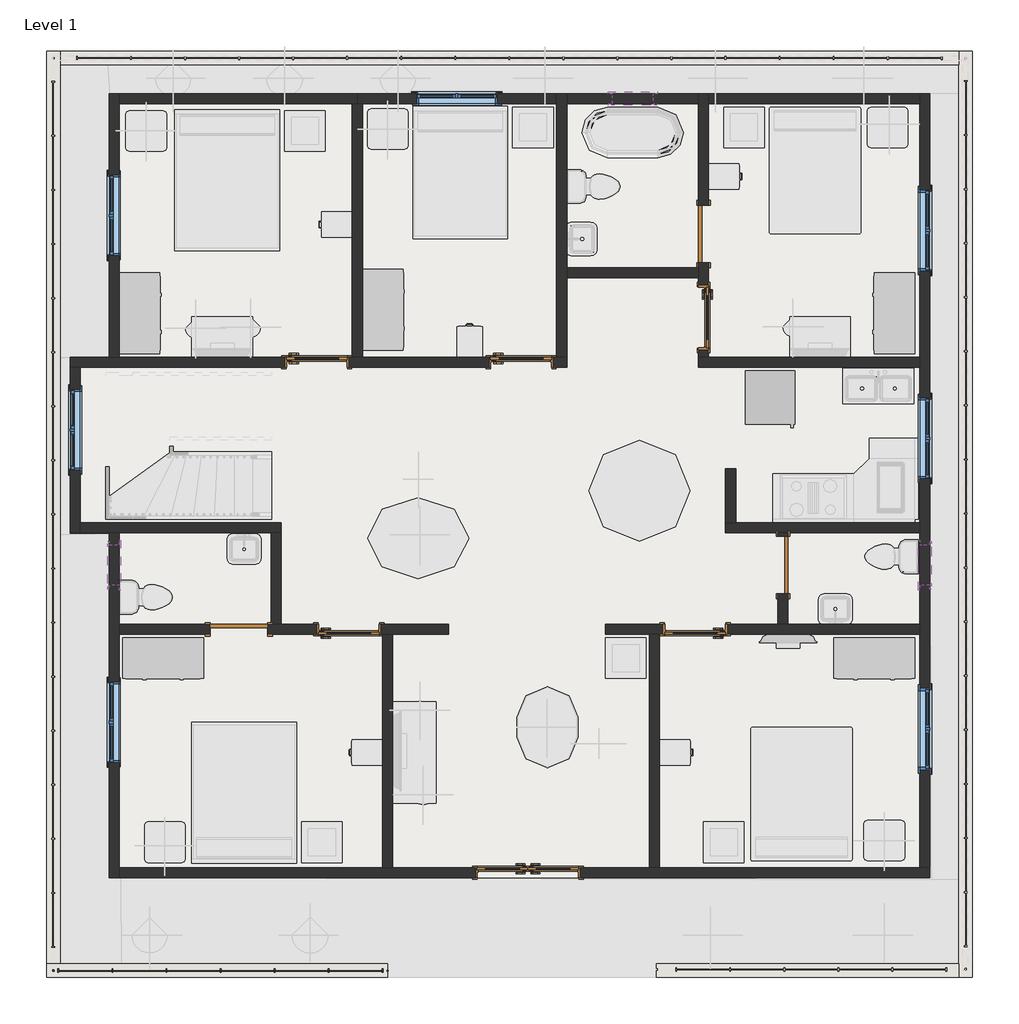
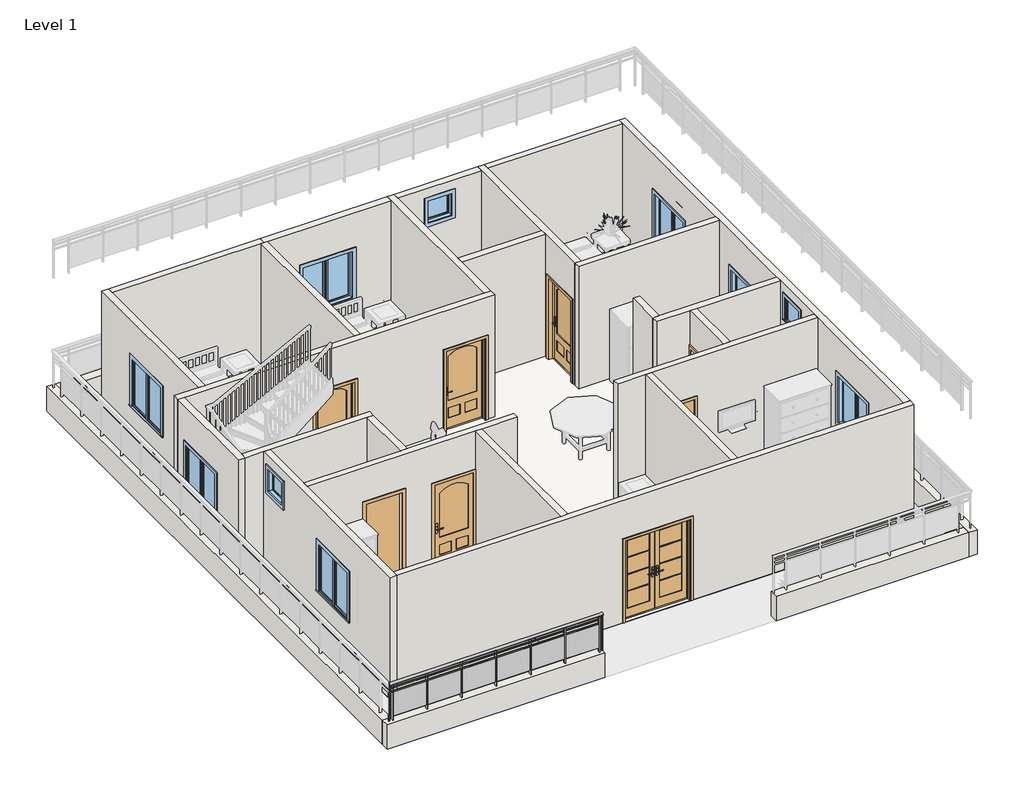
# One storey, part 1 of 5: 29 walls, 10 windows, 9 doors, 1 railing, 1 slab.
"""IFC4 building model written with IfcOpenShell, lengths in millimetres."""

from ifc_helpers import new_model, si_unit, point, frame, origin, origin_with_axes, place, context, project, spatial, polyline, ellipse_curve, trimmed, outline, extrude, faceted_brep, transform, mapped, element, save
from ifc_brep_helpers import plane_surface, extruded_surface, advanced_brep
from components import door_5d363d20, door_808aeb8e, door_94998e6c, door_99d96fc5, door_b6e9fca3, window_be30da88, window_3d781103

model = new_model("IFC4")

# Units and contexts
model_context = context("Model", 3, world=origin())
ifc_project = project(units=[si_unit("LENGTHUNIT", "METRE", prefix="MILLI")], contexts=[model_context])

# Site, building, storey
site = spatial("IfcSite", under=ifc_project)
building = spatial("IfcBuilding", under=site)
storey = spatial("IfcBuildingStorey", under=building, Name="Level 1", Elevation=0.0)

# Doors
placement = place(None, origin())
door_shape = door_5d363d20(model_context)
element("IfcDoor", 1, ObjectType="36\" x 80\"", at=placement, inside=storey, context=model_context, shape_type="MappedRepresentation", body=[
    mapped(door_shape, transform((-7516.6434666, 9773.3466937, 0.0), x_axis=(-1.0, 0.0, 0.0), y_axis=(0.0, -1.0, 0.0), z_axis=(0.0, 0.0, 1.0))),
])
element("IfcDoor", 2, ObjectType="36\" x 80\"", at=placement, inside=storey, context=model_context, shape_type="MappedRepresentation", body=[
    mapped(door_shape, transform((-4443.2434666, 9773.3466937, 0.0), x_axis=(-1.0, 0.0, 0.0), y_axis=(0.0, -1.0, 0.0), z_axis=(0.0, 0.0, 1.0))),
])
element("IfcDoor", 3, ObjectType="36\" x 80\"", at=placement, inside=storey, context=model_context, shape_type="MappedRepresentation", body=[
    mapped(door_shape, transform((-1696.8684666, 10443.2716937, 0.0), x_axis=(0.0, 1.0, 0.0), y_axis=(-1.0, 0.0, 0.0), z_axis=(0.0, 0.0, 1.0))),
])
element("IfcDoor", 4, ObjectType="36\" x 80\"", at=placement, inside=storey, context=model_context, shape_type="MappedRepresentation", body=[
    mapped(door_shape, transform((-1827.0434666, 5753.7966937, 0.0), x_axis=(1.0, 0.0, 0.0), y_axis=(0.0, 1.0, 0.0), z_axis=(0.0, 0.0, 1.0))),
])
door_2_shape = door_808aeb8e(model_context)
element("IfcDoor", 5, ObjectType="36\" x 80\"", at=placement, inside=storey, context=model_context, shape_type="MappedRepresentation", body=[
    mapped(door_2_shape, transform((-7034.0434666, 5753.7966937, 0.0), x_axis=(-1.0, 0.0, 0.0), y_axis=(0.0, -1.0, 0.0), z_axis=(0.0, 0.0, 1.0))),
])
door_3_shape = door_94998e6c(model_context)
element("IfcDoor", 6, ObjectType="Door-Exterior-Double-Full Glass-Wood_Clad : 60\" x 80\"", at=placement, inside=storey, context=model_context, shape_type="MappedRepresentation", body=[
    mapped(door_3_shape, transform((-4341.6434666, 2102.5466937, 0.0), x_axis=(1.0, 0.0, 0.0), y_axis=(0.0, 1.0, 0.0), z_axis=(0.0, 0.0, 1.0))),
])
door_4_shape = door_99d96fc5(model_context)
element("IfcDoor", 7, ObjectType="Single-Flush : 34\" x 84\"", at=placement, inside=storey, context=model_context, shape_type="MappedRepresentation", body=[
    mapped(door_4_shape, transform((-1700.0434666, 11700.5716937, 0.0), x_axis=(0.0, -1.0, 0.0), y_axis=(1.0, 0.0, 0.0), z_axis=(0.0, 0.0, 1.0))),
])
element("IfcDoor", 8, ObjectType="Single-Flush : 34\" x 84\"", at=placement, inside=storey, context=model_context, shape_type="MappedRepresentation", body=[
    mapped(door_4_shape, transform((-506.2434666, 6722.1716937, 0.0), x_axis=(0.0, 1.0, 0.0), y_axis=(-1.0, 0.0, 0.0), z_axis=(0.0, 0.0, 1.0))),
])
door_5_shape = door_b6e9fca3(model_context)
element("IfcDoor", 9, ObjectType="Single-Flush : 34\" x 84\"", at=placement, inside=storey, context=model_context, shape_type="MappedRepresentation", body=[
    mapped(door_5_shape, transform((-8685.0434666, 5756.9716937, 0.0), x_axis=(1.0, 0.0, 0.0), y_axis=(0.0, 1.0, 0.0), z_axis=(0.0, 0.0, 1.0))),
])

# Railing
element("IfcRailing", 10, ObjectType="Glass Panel - Bottom Fill", at=placement, inside=storey, context=model_context, shape_type="SolidModel", body=[
    advanced_brep(
    [(-6449.8434666, 588.0716937, 1524.0), (-6449.8434666, 664.2716937, 1524.0), (-11479.0434666, 588.0716937, 1524.0), (-11479.0434666, 664.2716937, 1524.0)],
    [
        (0, 1, ellipse_curve(frame((-6449.8434666, 626.1716937, 1524.0), z_axis=(1.0, 0.0, 0.0), x_axis=(0.0, 1.0, 0.0)), 38.1, 28.575)),
        (1, 0, ellipse_curve(frame((-6449.8434666, 626.1716937, 1524.0), z_axis=(1.0, 0.0, 0.0), x_axis=(0.0, 1.0, 0.0)), 38.1, 28.575)),
        (2, 3, ellipse_curve(frame((-11479.0434666, 626.1716937, 1524.0), z_axis=(-1.0, 0.0, 0.0), x_axis=(0.0, 1.0, 0.0)), 38.1, 28.575)),
        (3, 2, ellipse_curve(frame((-11479.0434666, 626.1716937, 1524.0), z_axis=(-1.0, 0.0, 0.0), x_axis=(0.0, 1.0, 0.0)), 38.1, 28.575)),
        (0, 2),
        (3, 1),
    ],
    [
        plane_surface(frame((-6449.8434666, 626.1716937, 1524.0), z_axis=(1.0, 0.0, 0.0), x_axis=(0.0, -1.0, 0.0))),
        plane_surface(frame((-11479.0434666, 626.1716937, 1524.0), z_axis=(-1.0, 0.0, 0.0), x_axis=(0.0, -1.0, 0.0))),
        extruded_surface(trimmed(ellipse_curve(frame((-11479.0434666, 626.1716937, 1524.0), z_axis=(1.0, 0.0, 0.0), x_axis=(0.0, 1.0, 0.0)), 38.1, 28.575), [point((-11479.0434666, 588.0716937, 1524.0))], [point((-11479.0434666, 664.2716937, 1524.0))], True, "CARTESIAN"), (5029.2, 0.0, 0.0), 5029.2),
        extruded_surface(trimmed(ellipse_curve(frame((-11479.0434666, 626.1716937, 1524.0), z_axis=(1.0, 0.0, 0.0), x_axis=(0.0, 1.0, 0.0)), 38.1, 28.575), [point((-11479.0434666, 664.2716937, 1524.0))], [point((-11479.0434666, 588.0716937, 1524.0))], True, "CARTESIAN"), (5029.2, 0.0, 0.0), 5029.2),
    ],
    [
        (0, [[1, 2]]),
        (1, [[3, 4]]),
        (2, [[-1, 5, -4, 6]]),
        (3, [[-2, -6, -3, -5]]),
    ],
),
    extrude(outline(polyline([(-6449.8434666, 638.8716937), (-6449.8434666, 613.4716937), (-11479.0434666, 613.4716937), (-11479.0434666, 638.8716937), (-6449.8434666, 638.8716937)])), frame((0.0, 0.0, 1409.7), z_axis=(0.0, 0.0, 1.0), x_axis=(1.0, 0.0, 0.0)), (0.0, 0.0, 1.0), 25.4),
    extrude(outline(polyline([(-6449.8434666, 638.8716937), (-6449.8434666, 613.4716937), (-11479.0434666, 613.4716937), (-11479.0434666, 638.8716937), (-6449.8434666, 638.8716937)])), frame((0.0, 0.0, 1308.1), z_axis=(0.0, 0.0, 1.0), x_axis=(1.0, 0.0, 0.0)), (0.0, 0.0, 1.0), 25.4),
    extrude(outline(polyline([(-11396.4934666, 651.5716937), (-11396.4934666, 600.7716937), (-11409.1934666, 600.7716937), (-11409.1934666, 651.5716937), (-11396.4934666, 651.5716937)])), frame((0.0, 0.0, 609.6), z_axis=(0.0, 0.0, 1.0), x_axis=(1.0, 0.0, 0.0)), (0.0, 0.0, 1.0), 885.6788223),
    extrude(outline(polyline([(-10590.0434666, 619.6365367), (-11402.8434666, 619.6365367), (-11402.8434666, 625.9865367), (-10590.0434666, 625.9865367), (-10590.0434666, 619.6365367)])), frame((0.0, 0.0, 711.2), z_axis=(0.0, 0.0, 1.0), x_axis=(1.0, 0.0, 0.0)), (0.0, 0.0, 1.0), 596.9),
    extrude(outline(polyline([(-10583.6934666, 651.5716937), (-10583.6934666, 600.7716937), (-10596.3934666, 600.7716937), (-10596.3934666, 651.5716937), (-10583.6934666, 651.5716937)])), frame((0.0, 0.0, 609.6), z_axis=(0.0, 0.0, 1.0), x_axis=(1.0, 0.0, 0.0)), (0.0, 0.0, 1.0), 885.6788223),
    extrude(outline(polyline([(-9777.2434666, 619.6365367), (-10590.0434666, 619.6365367), (-10590.0434666, 625.9865367), (-9777.2434666, 625.9865367), (-9777.2434666, 619.6365367)])), frame((0.0, 0.0, 711.2), z_axis=(0.0, 0.0, 1.0), x_axis=(1.0, 0.0, 0.0)), (0.0, 0.0, 1.0), 596.9),
    extrude(outline(polyline([(-9770.8934666, 651.5716937), (-9770.8934666, 600.7716937), (-9783.5934666, 600.7716937), (-9783.5934666, 651.5716937), (-9770.8934666, 651.5716937)])), frame((0.0, 0.0, 609.6), z_axis=(0.0, 0.0, 1.0), x_axis=(1.0, 0.0, 0.0)), (0.0, 0.0, 1.0), 885.6788223),
    extrude(outline(polyline([(-8964.4434666, 619.6365367), (-9777.2434666, 619.6365367), (-9777.2434666, 625.9865367), (-8964.4434666, 625.9865367), (-8964.4434666, 619.6365367)])), frame((0.0, 0.0, 711.2), z_axis=(0.0, 0.0, 1.0), x_axis=(1.0, 0.0, 0.0)), (0.0, 0.0, 1.0), 596.9),
    extrude(outline(polyline([(-8958.0934666, 651.5716937), (-8958.0934666, 600.7716937), (-8970.7934666, 600.7716937), (-8970.7934666, 651.5716937), (-8958.0934666, 651.5716937)])), frame((0.0, 0.0, 609.6), z_axis=(0.0, 0.0, 1.0), x_axis=(1.0, 0.0, 0.0)), (0.0, 0.0, 1.0), 885.6788223),
    extrude(outline(polyline([(-8151.6434666, 619.6365367), (-8964.4434666, 619.6365367), (-8964.4434666, 625.9865367), (-8151.6434666, 625.9865367), (-8151.6434666, 619.6365367)])), frame((0.0, 0.0, 711.2), z_axis=(0.0, 0.0, 1.0), x_axis=(1.0, 0.0, 0.0)), (0.0, 0.0, 1.0), 596.9),
    extrude(outline(polyline([(-8145.2934666, 651.5716937), (-8145.2934666, 600.7716937), (-8157.9934666, 600.7716937), (-8157.9934666, 651.5716937), (-8145.2934666, 651.5716937)])), frame((0.0, 0.0, 609.6), z_axis=(0.0, 0.0, 1.0), x_axis=(1.0, 0.0, 0.0)), (0.0, 0.0, 1.0), 885.6788223),
    extrude(outline(polyline([(-7338.8434666, 619.6365367), (-8151.6434666, 619.6365367), (-8151.6434666, 625.9865367), (-7338.8434666, 625.9865367), (-7338.8434666, 619.6365367)])), frame((0.0, 0.0, 711.2), z_axis=(0.0, 0.0, 1.0), x_axis=(1.0, 0.0, 0.0)), (0.0, 0.0, 1.0), 596.9),
    extrude(outline(polyline([(-7332.4934666, 651.5716937), (-7332.4934666, 600.7716937), (-7345.1934666, 600.7716937), (-7345.1934666, 651.5716937), (-7332.4934666, 651.5716937)])), frame((0.0, 0.0, 609.6), z_axis=(0.0, 0.0, 1.0), x_axis=(1.0, 0.0, 0.0)), (0.0, 0.0, 1.0), 885.6788223),
    extrude(outline(polyline([(-6526.0434666, 619.6365367), (-7338.8434666, 619.6365367), (-7338.8434666, 625.9865367), (-6526.0434666, 625.9865367), (-6526.0434666, 619.6365367)])), frame((0.0, 0.0, 711.2), z_axis=(0.0, 0.0, 1.0), x_axis=(1.0, 0.0, 0.0)), (0.0, 0.0, 1.0), 596.9),
    extrude(outline(polyline([(-6519.6934666, 651.5716937), (-6519.6934666, 600.7716937), (-6532.3934666, 600.7716937), (-6532.3934666, 651.5716937), (-6519.6934666, 651.5716937)])), frame((0.0, 0.0, 609.6), z_axis=(0.0, 0.0, 1.0), x_axis=(1.0, 0.0, 0.0)), (0.0, 0.0, 1.0), 885.6788223),
    extrude(outline(polyline([(-11466.3434666, 635.6966937), (-11466.3434666, 616.6466937), (-11485.3934666, 616.6466937), (-11485.3934666, 635.6966937), (-11466.3434666, 635.6966937)])), frame((0.0, 0.0, 609.6), z_axis=(0.0, 0.0, 1.0), x_axis=(1.0, 0.0, 0.0)), (0.0, 0.0, 1.0), 885.6788223),
    extrude(outline(polyline([(-6443.4934666, 635.6966937), (-6443.4934666, 616.6466937), (-6462.5434666, 616.6466937), (-6462.5434666, 635.6966937), (-6443.4934666, 635.6966937)])), frame((0.0, 0.0, 609.6), z_axis=(0.0, 0.0, 1.0), x_axis=(1.0, 0.0, 0.0)), (0.0, 0.0, 1.0), 885.6788223),
])

# Slab
element("IfcSlab", 11, ObjectType="Generic - 12\"", at=placement, inside=storey, context=model_context, shape_type="SweptSolid", body=[
    extrude(outline(polyline([(1703.5565334, 13808.7716937), (1703.5565334, 2023.1716937), (-10640.8434666, 2023.1716937), (-10640.8434666, 7204.7716937), (-11225.0434666, 7204.7716937), (-11225.0434666, 9846.3716937), (-10640.8434666, 9846.3716937), (-10640.8434666, 13808.7716937), (1703.5565334, 13808.7716937)])), frame((0.0, 0.0, -304.8), z_axis=(0.0, 0.0, 1.0), x_axis=(1.0, 0.0, 0.0)), (0.0, 0.0, 1.0), 304.8),
])

# Walls
element("IfcWall", 12, ObjectType="Generic - 5'", at=placement, inside=storey, context=model_context, shape_type="Brep", body=[
    faceted_brep([(2135.3565334, 14443.7716937, 0.0), (2135.3565334, 14240.5716937, 0.0), (2135.3565334, 727.7716937, 0.0), (2135.3565334, 524.5716937, 0.0), (2135.3565334, 524.5716937, 609.6), (2135.3565334, 727.7716937, 609.6), (2135.3565334, 14240.5716937, 609.6), (2135.3565334, 14443.7716937, 609.6), (2338.5565334, 14443.7716937, 0.0), (2338.5565334, 14443.7716937, 609.6), (2338.5565334, 524.5716937, 609.6), (2338.5565334, 524.5716937, 0.0)], [[[0, 1, 2, 3, 4, 5, 6, 7]], [[8, 9, 10, 11]], [[3, 2, 1, 0, 8, 11]], [[7, 6, 5, 4, 10, 9]], [[4, 3, 11, 10]], [[0, 7, 9, 8]]]),
])
element("IfcWall", 13, ObjectType="Generic - 5'", at=placement, inside=storey, context=model_context, shape_type="SweptSolid", body=[
    extrude(outline(polyline([(-2411.2434666, 727.7716937), (2135.3565334, 727.7716937), (2135.3565334, 524.5716937), (-2411.2434666, 524.5716937), (-2411.2434666, 727.7716937)])), origin_with_axes(), (0.0, 0.0, 1.0), 609.6),
])
element("IfcWall", 14, ObjectType="Generic - 5'", at=placement, inside=storey, context=model_context, shape_type="Brep", body=[
    faceted_brep([(-11377.4434666, 727.7716937, 0.0), (-11377.4434666, 14240.5716937, 0.0), (-11377.4434666, 14443.7716937, 0.0), (-11377.4434666, 14443.7716937, 609.6), (-11377.4434666, 14240.5716937, 609.6), (-11377.4434666, 727.7716937, 609.6), (-11580.6434666, 727.7716937, 0.0), (-11580.6434666, 727.7716937, 609.6), (-11580.6434666, 14443.7716937, 609.6), (-11580.6434666, 14443.7716937, 0.0)], [[[0, 1, 2, 3, 4, 5]], [[6, 7, 8, 9]], [[2, 1, 0, 6, 9]], [[5, 4, 3, 8, 7]], [[0, 5, 7, 6]], [[3, 2, 9, 8]]]),
])
element("IfcWall", 15, ObjectType="Generic - 5'", at=placement, inside=storey, context=model_context, shape_type="SweptSolid", body=[
    extrude(outline(polyline([(2135.3565334, 14240.5716937), (-11377.4434666, 14240.5716937), (-11377.4434666, 14443.7716937), (2135.3565334, 14443.7716937), (2135.3565334, 14240.5716937)])), origin_with_axes(), (0.0, 0.0, 1.0), 609.6),
])
element("IfcWall", 16, ObjectType="Generic - 5'", at=placement, inside=storey, context=model_context, shape_type="Brep", body=[
    faceted_brep([(-6449.8434666, 727.7716937, 0.0), (-11377.4434666, 727.7716937, 0.0), (-11580.6434666, 727.7716937, 0.0), (-11580.6434666, 727.7716937, 609.6), (-11377.4434666, 727.7716937, 609.6), (-6449.8434666, 727.7716937, 609.6), (-6449.8434666, 524.5716937, 0.0), (-6449.8434666, 524.5716937, 609.6), (-11580.6434666, 524.5716937, 609.6), (-11580.6434666, 524.5716937, 0.0)], [[[0, 1, 2, 3, 4, 5]], [[6, 7, 8, 9]], [[2, 1, 0, 6, 9]], [[5, 4, 3, 8, 7]], [[0, 5, 7, 6]], [[3, 2, 9, 8]]]),
])
element("IfcWall", 17, ObjectType="INNER WALL 6\"", at=placement, inside=storey, context=model_context, shape_type="Brep", body=[
    faceted_brep([(-11225.0434666, 9693.9716937, 3048.0), (-11225.0434666, 9693.9716937, 0.0), (-11072.6434666, 9693.9716937, 0.0), (-7999.2434666, 9693.9716937, 0.0), (-7999.2434666, 9693.9716937, 2057.4), (-7034.0434666, 9693.9716937, 2057.4), (-7034.0434666, 9693.9716937, 0.0), (-4925.8434666, 9693.9716937, 0.0), (-4925.8434666, 9693.9716937, 2057.4), (-3960.6434666, 9693.9716937, 2057.4), (-3960.6434666, 9693.9716937, 0.0), (-3757.4434666, 9693.9716937, 0.0), (-3757.4434666, 9693.9716937, 3048.0), (-11072.6434666, 9693.9716937, 3048.0), (-11225.0434666, 9846.3716937, 0.0), (-11225.0434666, 9846.3716937, 3048.0), (-10640.8434666, 9846.3716937, 3048.0), (-10488.4434666, 9846.3716937, 3048.0), (-6983.2434666, 9846.3716937, 3048.0), (-6830.8434666, 9846.3716937, 3048.0), (-3909.8434666, 9846.3716937, 3048.0), (-3757.4434666, 9846.3716937, 3048.0), (-3757.4434666, 9846.3716937, 0.0), (-3909.8434666, 9846.3716937, 0.0), (-3960.6434666, 9846.3716937, 0.0), (-3960.6434666, 9846.3716937, 2057.4), (-4925.8434666, 9846.3716937, 2057.4), (-4925.8434666, 9846.3716937, 0.0), (-6830.8434666, 9846.3716937, 0.0), (-6983.2434666, 9846.3716937, 0.0), (-7034.0434666, 9846.3716937, 0.0), (-7034.0434666, 9846.3716937, 2057.4), (-7999.2434666, 9846.3716937, 2057.4), (-7999.2434666, 9846.3716937, 0.0), (-10488.4434666, 9846.3716937, 0.0), (-10640.8434666, 9846.3716937, 0.0)], [[[0, 1, 2, 3, 4, 5, 6, 7, 8, 9, 10, 11, 12, 13]], [[14, 15, 16, 17, 18, 19, 20, 21, 22, 23, 24, 25, 26, 27, 28, 29, 30, 31, 32, 33, 34, 35]], [[1, 14, 35, 34, 33, 3, 2]], [[22, 11, 10, 24, 23]], [[6, 30, 29, 28, 27, 7]], [[1, 0, 15, 14]], [[12, 11, 22, 21]], [[32, 4, 3, 33]], [[4, 32, 31, 5]], [[5, 31, 30, 6]], [[26, 8, 7, 27]], [[8, 26, 25, 9]], [[9, 25, 24, 10]], [[0, 13, 12, 21, 20, 19, 18, 17, 16, 15]]]),
])
element("IfcWall", 18, ObjectType="INNER WALL 6\"", at=placement, inside=storey, context=model_context, shape_type="Brep", body=[
    faceted_brep([(-10488.4434666, 13656.3716937, 0.0), (-6983.2434666, 13656.3716937, 0.0), (-6907.0434666, 13656.3716937, 0.0), (-6907.0434666, 13656.3716937, 3048.0), (-6983.2434666, 13656.3716937, 3048.0), (-10488.4434666, 13656.3716937, 3048.0), (-10488.4434666, 13808.7716937, 0.0), (-10488.4434666, 13808.7716937, 3048.0), (-6907.0434666, 13808.7716937, 3048.0), (-6907.0434666, 13808.7716937, 0.0)], [[[0, 1, 2, 3, 4, 5]], [[6, 7, 8, 9]], [[2, 1, 0, 6, 9]], [[3, 2, 9, 8]], [[0, 5, 7, 6]], [[5, 4, 3, 8, 7]]]),
])
element("IfcWall", 19, ObjectType="INNER WALL 6\"", at=placement, inside=storey, context=model_context, shape_type="Brep", body=[
    faceted_brep([(-10640.8434666, 13808.7716937, 0.0), (-10640.8434666, 9846.3716937, 0.0), (-10640.8434666, 9846.3716937, 3048.0), (-10640.8434666, 13808.7716937, 3048.0), (-10640.8434666, 12589.5716937, 2133.6), (-10640.8434666, 11370.3716937, 2133.6), (-10640.8434666, 11370.3716937, 914.4), (-10640.8434666, 12589.5716937, 914.4), (-10488.4434666, 13808.7716937, 0.0), (-10488.4434666, 13808.7716937, 3048.0), (-10488.4434666, 13656.3716937, 3048.0), (-10488.4434666, 9846.3716937, 3048.0), (-10488.4434666, 9846.3716937, 0.0), (-10488.4434666, 13656.3716937, 0.0), (-10488.4434666, 12589.5716937, 2133.6), (-10488.4434666, 12589.5716937, 914.4), (-10488.4434666, 11370.3716937, 914.4), (-10488.4434666, 11370.3716937, 2133.6)], [[[0, 1, 2, 3], [4, 5, 6, 7]], [[8, 9, 10, 11, 12, 13], [14, 15, 16, 17]], [[1, 0, 8, 13, 12]], [[2, 1, 12, 11]], [[0, 3, 9, 8]], [[15, 14, 4, 7]], [[16, 15, 7, 6]], [[17, 16, 6, 5]], [[14, 17, 5, 4]], [[3, 2, 11, 10, 9]]]),
])
element("IfcWall", 20, ObjectType="INNER WALL 6\"", at=placement, inside=storey, context=model_context, shape_type="Brep", body=[
    faceted_brep([(-6907.0434666, 13656.3716937, 0.0), (-6830.8434666, 13656.3716937, 0.0), (-3909.8434666, 13656.3716937, 0.0), (-3909.8434666, 13656.3716937, 3048.0), (-6830.8434666, 13656.3716937, 3048.0), (-6907.0434666, 13656.3716937, 3048.0), (-4798.8434666, 13656.3716937, 2133.6), (-4798.8434666, 13656.3716937, 914.4), (-6018.0434666, 13656.3716937, 914.4), (-6018.0434666, 13656.3716937, 2133.6), (-6907.0434666, 13808.7716937, 0.0), (-6907.0434666, 13808.7716937, 3048.0), (-3909.8434666, 13808.7716937, 3048.0), (-3909.8434666, 13808.7716937, 0.0), (-4798.8434666, 13808.7716937, 2133.6), (-6018.0434666, 13808.7716937, 2133.6), (-6018.0434666, 13808.7716937, 914.4), (-4798.8434666, 13808.7716937, 914.4)], [[[0, 1, 2, 3, 4, 5], [6, 7, 8, 9]], [[10, 11, 12, 13], [14, 15, 16, 17]], [[2, 1, 0, 10, 13]], [[0, 5, 11, 10]], [[3, 2, 13, 12]], [[7, 6, 14, 17]], [[8, 7, 17, 16]], [[9, 8, 16, 15]], [[6, 9, 15, 14]], [[5, 4, 3, 12, 11]]]),
])
element("IfcWall", 21, ObjectType="INNER WALL 6\"", at=placement, inside=storey, context=model_context, shape_type="Brep", body=[
    faceted_brep([(-6983.2434666, 13656.3716937, 0.0), (-6983.2434666, 9846.3716937, 0.0), (-6983.2434666, 9846.3716937, 3048.0), (-6983.2434666, 13656.3716937, 3048.0), (-6830.8434666, 13656.3716937, 0.0), (-6830.8434666, 13656.3716937, 3048.0), (-6830.8434666, 9846.3716937, 3048.0), (-6830.8434666, 9846.3716937, 0.0), (-6907.0434666, 13656.3716937, 0.0), (-6907.0434666, 13656.3716937, 3048.0)], [[[0, 1, 2, 3]], [[4, 5, 6, 7]], [[1, 0, 8, 4, 7]], [[2, 1, 7, 6]], [[0, 3, 9, 5, 4, 8]], [[3, 2, 6, 5, 9]]]),
])
element("IfcWall", 22, ObjectType="INNER WALL 6\"", at=placement, inside=storey, context=model_context, shape_type="SweptSolid", body=[
    extrude(outline(polyline([(0.0, -3757.4434666), (0.0, -1776.2434666), (3048.0, -1776.2434666), (3048.0, -3757.4434666), (0.0, -3757.4434666)]), holes=[polyline([(2768.6, -2462.0434666), (2159.0, -2462.0434666), (2159.0, -3071.6434666), (2768.6, -3071.6434666), (2768.6, -2462.0434666)])]), frame((0.0, 13656.3716937, 0.0), z_axis=(0.0, 1.0, 0.0), x_axis=(0.0, 0.0, 1.0)), (0.0, 0.0, 1.0), 152.4),
])
element("IfcWall", 23, ObjectType="INNER WALL 6\"", at=placement, inside=storey, context=model_context, shape_type="Brep", body=[
    faceted_brep([(-3909.8434666, 13808.7716937, 0.0), (-3909.8434666, 13656.3716937, 0.0), (-3909.8434666, 9846.3716937, 0.0), (-3909.8434666, 9846.3716937, 3048.0), (-3909.8434666, 13656.3716937, 3048.0), (-3909.8434666, 13808.7716937, 3048.0), (-3757.4434666, 13808.7716937, 0.0), (-3757.4434666, 13808.7716937, 3048.0), (-3757.4434666, 13656.3716937, 3048.0), (-3757.4434666, 11192.5716937, 3048.0), (-3757.4434666, 11040.1716937, 3048.0), (-3757.4434666, 9846.3716937, 3048.0), (-3757.4434666, 9846.3716937, 0.0), (-3757.4434666, 11040.1716937, 0.0), (-3757.4434666, 11192.5716937, 0.0), (-3757.4434666, 13656.3716937, 0.0)], [[[0, 1, 2, 3, 4, 5]], [[6, 7, 8, 9, 10, 11, 12, 13, 14, 15]], [[2, 1, 0, 6, 15, 14, 13, 12]], [[3, 2, 12, 11]], [[0, 5, 7, 6]], [[5, 4, 3, 11, 10, 9, 8, 7]]]),
])
element("IfcWall", 24, ObjectType="INNER WALL 6\"", at=placement, inside=storey, context=model_context, shape_type="SweptSolid", body=[
    extrude(outline(polyline([(1551.1565334, 13656.3716937), (-1623.8434666, 13656.3716937), (-1623.8434666, 13808.7716937), (1551.1565334, 13808.7716937), (1551.1565334, 13656.3716937)])), origin_with_axes(), (0.0, 0.0, 1.0), 3048.0),
])
element("IfcWall", 25, ObjectType="INNER WALL 6\"", at=placement, inside=storey, context=model_context, shape_type="Brep", body=[
    faceted_brep([(-1776.2434666, 11268.7716937, 2133.6), (-1776.2434666, 11268.7716937, 0.0), (-1776.2434666, 11192.5716937, 0.0), (-1776.2434666, 11040.1716937, 0.0), (-1776.2434666, 10925.8716937, 0.0), (-1776.2434666, 10925.8716937, 2057.4), (-1776.2434666, 9960.6716937, 2057.4), (-1776.2434666, 9960.6716937, 0.0), (-1776.2434666, 9846.3716937, 0.0), (-1776.2434666, 9846.3716937, 3048.0), (-1776.2434666, 11040.1716937, 3048.0), (-1776.2434666, 11192.5716937, 3048.0), (-1776.2434666, 13656.3716937, 3048.0), (-1776.2434666, 13808.7716937, 3048.0), (-1776.2434666, 13808.7716937, 0.0), (-1776.2434666, 13656.3716937, 0.0), (-1776.2434666, 12132.3716937, 0.0), (-1776.2434666, 12132.3716937, 2133.6), (-1623.8434666, 10925.8716937, 0.0), (-1623.8434666, 11268.7716937, 0.0), (-1623.8434666, 11268.7716937, 2133.6), (-1623.8434666, 12132.3716937, 2133.6), (-1623.8434666, 12132.3716937, 0.0), (-1623.8434666, 13656.3716937, 0.0), (-1623.8434666, 13808.7716937, 0.0), (-1623.8434666, 13808.7716937, 3048.0), (-1623.8434666, 13656.3716937, 3048.0), (-1623.8434666, 9846.3716937, 3048.0), (-1623.8434666, 9846.3716937, 0.0), (-1623.8434666, 9960.6716937, 0.0), (-1623.8434666, 9960.6716937, 2057.4), (-1623.8434666, 10925.8716937, 2057.4)], [[[0, 1, 2, 3, 4, 5, 6, 7, 8, 9, 10, 11, 12, 13, 14, 15, 16, 17]], [[18, 19, 20, 21, 22, 23, 24, 25, 26, 27, 28, 29, 30, 31]], [[28, 8, 7, 29]], [[16, 15, 14, 24, 23, 22]], [[4, 3, 2, 1, 19, 18]], [[9, 8, 28, 27]], [[14, 13, 25, 24]], [[31, 5, 4, 18]], [[5, 31, 30, 6]], [[6, 30, 29, 7]], [[20, 19, 1, 0]], [[21, 20, 0, 17]], [[22, 21, 17, 16]], [[13, 12, 11, 10, 9, 27, 26, 25]]]),
])
element("IfcWall", 26, ObjectType="INNER WALL 6\"", at=placement, inside=storey, context=model_context, shape_type="Brep", body=[
    faceted_brep([(1551.1565334, 13808.7716937, 0.0), (1551.1565334, 13656.3716937, 0.0), (1551.1565334, 9846.3716937, 0.0), (1551.1565334, 9693.9716937, 0.0), (1551.1565334, 7357.1716937, 0.0), (1551.1565334, 7204.7716937, 0.0), (1551.1565334, 5833.1716937, 0.0), (1551.1565334, 5680.7716937, 0.0), (1551.1565334, 2175.5716937, 0.0), (1551.1565334, 2175.5716937, 3048.0), (1551.1565334, 5680.7716937, 3048.0), (1551.1565334, 5833.1716937, 3048.0), (1551.1565334, 7204.7716937, 3048.0), (1551.1565334, 7357.1716937, 3048.0), (1551.1565334, 9693.9716937, 3048.0), (1551.1565334, 9846.3716937, 3048.0), (1551.1565334, 13656.3716937, 3048.0), (1551.1565334, 13808.7716937, 3048.0), (1551.1565334, 11141.7716937, 2133.6), (1551.1565334, 11141.7716937, 914.4), (1551.1565334, 12360.9716937, 914.4), (1551.1565334, 12360.9716937, 2133.6), (1551.1565334, 8017.5716937, 2133.6), (1551.1565334, 8017.5716937, 914.4), (1551.1565334, 9236.7716937, 914.4), (1551.1565334, 9236.7716937, 2133.6), (1551.1565334, 3648.7716937, 2133.6), (1551.1565334, 3648.7716937, 914.4), (1551.1565334, 4867.9716937, 914.4), (1551.1565334, 4867.9716937, 2133.6), (1551.1565334, 7026.9716937, 2768.6), (1551.1565334, 6417.3716937, 2768.6), (1551.1565334, 6417.3716937, 2159.0), (1551.1565334, 7026.9716937, 2159.0), (1703.5565334, 13808.7716937, 0.0), (1703.5565334, 13808.7716937, 3048.0), (1703.5565334, 2175.5716937, 3048.0), (1703.5565334, 2175.5716937, 0.0), (1703.5565334, 11141.7716937, 2133.6), (1703.5565334, 12360.9716937, 2133.6), (1703.5565334, 12360.9716937, 914.4), (1703.5565334, 11141.7716937, 914.4), (1703.5565334, 8017.5716937, 2133.6), (1703.5565334, 9236.7716937, 2133.6), (1703.5565334, 9236.7716937, 914.4), (1703.5565334, 8017.5716937, 914.4), (1703.5565334, 3648.7716937, 2133.6), (1703.5565334, 4867.9716937, 2133.6), (1703.5565334, 4867.9716937, 914.4), (1703.5565334, 3648.7716937, 914.4), (1703.5565334, 7026.9716937, 2768.6), (1703.5565334, 7026.9716937, 2159.0), (1703.5565334, 6417.3716937, 2159.0), (1703.5565334, 6417.3716937, 2768.6)], [[[0, 1, 2, 3, 4, 5, 6, 7, 8, 9, 10, 11, 12, 13, 14, 15, 16, 17], [18, 19, 20, 21], [22, 23, 24, 25], [26, 27, 28, 29], [30, 31, 32, 33]], [[34, 35, 36, 37], [38, 39, 40, 41], [42, 43, 44, 45], [46, 47, 48, 49], [50, 51, 52, 53]], [[8, 7, 6, 5, 4, 3, 2, 1, 0, 34, 37]], [[0, 17, 35, 34]], [[9, 8, 37, 36]], [[19, 18, 38, 41]], [[20, 19, 41, 40]], [[21, 20, 40, 39]], [[18, 21, 39, 38]], [[23, 22, 42, 45]], [[24, 23, 45, 44]], [[25, 24, 44, 43]], [[22, 25, 43, 42]], [[27, 26, 46, 49]], [[28, 27, 49, 48]], [[29, 28, 48, 47]], [[26, 29, 47, 46]], [[51, 50, 30, 33]], [[52, 51, 33, 32]], [[53, 52, 32, 31]], [[50, 53, 31, 30]], [[17, 16, 15, 14, 13, 12, 11, 10, 9, 36, 35]]]),
])
element("IfcWall", 27, ObjectType="INNER WALL 6\"", at=placement, inside=storey, context=model_context, shape_type="Brep", body=[
    faceted_brep([(-11225.0434666, 9693.9716937, 0.0), (-11225.0434666, 7204.7716937, 0.0), (-11225.0434666, 7204.7716937, 3048.0), (-11225.0434666, 9693.9716937, 3048.0), (-11225.0434666, 9363.7716937, 2133.6), (-11225.0434666, 8144.5716937, 2133.6), (-11225.0434666, 8144.5716937, 914.4), (-11225.0434666, 9363.7716937, 914.4), (-11072.6434666, 9693.9716937, 0.0), (-11072.6434666, 9693.9716937, 3048.0), (-11072.6434666, 7357.1716937, 3048.0), (-11072.6434666, 7204.7716937, 3048.0), (-11072.6434666, 7204.7716937, 0.0), (-11072.6434666, 7357.1716937, 0.0), (-11072.6434666, 9363.7716937, 2133.6), (-11072.6434666, 9363.7716937, 914.4), (-11072.6434666, 8144.5716937, 914.4), (-11072.6434666, 8144.5716937, 2133.6)], [[[0, 1, 2, 3], [4, 5, 6, 7]], [[8, 9, 10, 11, 12, 13], [14, 15, 16, 17]], [[1, 0, 8, 13, 12]], [[0, 3, 9, 8]], [[2, 1, 12, 11]], [[15, 14, 4, 7]], [[16, 15, 7, 6]], [[17, 16, 6, 5]], [[14, 17, 5, 4]], [[3, 2, 11, 10, 9]]]),
])
element("IfcWall", 28, ObjectType="INNER WALL 6\"", at=placement, inside=storey, context=model_context, shape_type="Brep", body=[
    faceted_brep([(-11072.6434666, 7204.7716937, 0.0), (-10640.8434666, 7204.7716937, 0.0), (-10488.4434666, 7204.7716937, 0.0), (-8202.4434666, 7204.7716937, 0.0), (-8050.0434666, 7204.7716937, 0.0), (-8050.0434666, 7204.7716937, 3048.0), (-8202.4434666, 7204.7716937, 3048.0), (-10488.4434666, 7204.7716937, 3048.0), (-10640.8434666, 7204.7716937, 3048.0), (-11072.6434666, 7204.7716937, 3048.0), (-11072.6434666, 7357.1716937, 0.0), (-11072.6434666, 7357.1716937, 3048.0), (-8050.0434666, 7357.1716937, 3048.0), (-8050.0434666, 7357.1716937, 0.0)], [[[0, 1, 2, 3, 4, 5, 6, 7, 8, 9]], [[10, 11, 12, 13]], [[4, 3, 2, 1, 0, 10, 13]], [[0, 9, 11, 10]], [[5, 4, 13, 12]], [[9, 8, 7, 6, 5, 12, 11]]]),
])
element("IfcWall", 29, ObjectType="INNER WALL 6\"", at=placement, inside=storey, context=model_context, shape_type="SweptSolid", body=[
    extrude(outline(polyline([(-8202.4434666, 5833.1716937), (-8202.4434666, 7204.7716937), (-8050.0434666, 7204.7716937), (-8050.0434666, 5833.1716937), (-8202.4434666, 5833.1716937)])), origin_with_axes(), (0.0, 0.0, 1.0), 3048.0),
])
element("IfcWall", 30, ObjectType="INNER WALL 6\"", at=placement, inside=storey, context=model_context, shape_type="Brep", body=[
    faceted_brep([(-3173.2434666, 5833.1716937, 0.0), (-3173.2434666, 5833.1716937, 3048.0), (-582.4434666, 5833.1716937, 3048.0), (-430.0434666, 5833.1716937, 3048.0), (1551.1565334, 5833.1716937, 3048.0), (1551.1565334, 5833.1716937, 0.0), (-430.0434666, 5833.1716937, 0.0), (-582.4434666, 5833.1716937, 0.0), (-1344.4434666, 5833.1716937, 0.0), (-1344.4434666, 5833.1716937, 2057.4), (-2309.6434666, 5833.1716937, 2057.4), (-2309.6434666, 5833.1716937, 0.0), (-3173.2434666, 5680.7716937, 3048.0), (-3173.2434666, 5680.7716937, 0.0), (-2512.8434666, 5680.7716937, 0.0), (-2360.4434666, 5680.7716937, 0.0), (-2309.6434666, 5680.7716937, 0.0), (-2309.6434666, 5680.7716937, 2057.4), (-1344.4434666, 5680.7716937, 2057.4), (-1344.4434666, 5680.7716937, 0.0), (1551.1565334, 5680.7716937, 0.0), (1551.1565334, 5680.7716937, 3048.0), (-2360.4434666, 5680.7716937, 3048.0), (-2512.8434666, 5680.7716937, 3048.0)], [[[0, 1, 2, 3, 4, 5, 6, 7, 8, 9, 10, 11]], [[12, 13, 14, 15, 16, 17, 18, 19, 20, 21, 22, 23]], [[13, 0, 11, 16, 15, 14]], [[5, 20, 19, 8, 7, 6]], [[1, 0, 13, 12]], [[5, 4, 21, 20]], [[18, 9, 8, 19]], [[9, 18, 17, 10]], [[10, 17, 16, 11]], [[4, 3, 2, 1, 12, 23, 22, 21]]]),
])
element("IfcWall", 31, ObjectType="INNER WALL 6\"", at=placement, inside=storey, context=model_context, shape_type="Brep", body=[
    faceted_brep([(-10488.4434666, 2023.1716937, 0.0), (-10488.4434666, 2175.5716937, 0.0), (-10488.4434666, 5680.7716937, 0.0), (-10488.4434666, 5833.1716937, 0.0), (-10488.4434666, 7204.7716937, 0.0), (-10488.4434666, 7204.7716937, 3048.0), (-10488.4434666, 5833.1716937, 3048.0), (-10488.4434666, 5680.7716937, 3048.0), (-10488.4434666, 2175.5716937, 3048.0), (-10488.4434666, 2023.1716937, 3048.0), (-10488.4434666, 4969.5716937, 2133.6), (-10488.4434666, 4969.5716937, 914.4), (-10488.4434666, 3750.3716937, 914.4), (-10488.4434666, 3750.3716937, 2133.6), (-10488.4434666, 6417.3716937, 2768.6), (-10488.4434666, 7026.9716937, 2768.6), (-10488.4434666, 7026.9716937, 2159.0), (-10488.4434666, 6417.3716937, 2159.0), (-10640.8434666, 2023.1716937, 0.0), (-10640.8434666, 2023.1716937, 3048.0), (-10640.8434666, 7204.7716937, 3048.0), (-10640.8434666, 7204.7716937, 0.0), (-10640.8434666, 4969.5716937, 2133.6), (-10640.8434666, 3750.3716937, 2133.6), (-10640.8434666, 3750.3716937, 914.4), (-10640.8434666, 4969.5716937, 914.4), (-10640.8434666, 6417.3716937, 2768.6), (-10640.8434666, 6417.3716937, 2159.0), (-10640.8434666, 7026.9716937, 2159.0), (-10640.8434666, 7026.9716937, 2768.6)], [[[0, 1, 2, 3, 4, 5, 6, 7, 8, 9], [10, 11, 12, 13], [14, 15, 16, 17]], [[18, 19, 20, 21], [22, 23, 24, 25], [26, 27, 28, 29]], [[4, 3, 2, 1, 0, 18, 21]], [[5, 4, 21, 20]], [[0, 9, 19, 18]], [[11, 10, 22, 25]], [[12, 11, 25, 24]], [[13, 12, 24, 23]], [[10, 13, 23, 22]], [[27, 26, 14, 17]], [[28, 27, 17, 16]], [[29, 28, 16, 15]], [[26, 29, 15, 14]], [[9, 8, 7, 6, 5, 20, 19]]]),
])
element("IfcWall", 32, ObjectType="INNER WALL 6\"", at=placement, inside=storey, context=model_context, shape_type="Brep", body=[
    faceted_brep([(-10488.4434666, 2023.1716937, 3048.0), (-10488.4434666, 2023.1716937, 0.0), (-5129.0434666, 2023.1716937, 0.0), (-5129.0434666, 2023.1716937, 2057.4), (-3554.2434666, 2023.1716937, 2057.4), (-3554.2434666, 2023.1716937, 0.0), (1703.5565334, 2023.1716937, 0.0), (1703.5565334, 2023.1716937, 3048.0), (-10488.4434666, 2175.5716937, 0.0), (-10488.4434666, 2175.5716937, 3048.0), (-6526.0434666, 2175.5716937, 3048.0), (-6373.6434666, 2175.5716937, 3048.0), (-2512.8434666, 2175.5716937, 3048.0), (-2360.4434666, 2175.5716937, 3048.0), (1551.1565334, 2175.5716937, 3048.0), (1703.5565334, 2175.5716937, 3048.0), (1703.5565334, 2175.5716937, 0.0), (1551.1565334, 2175.5716937, 0.0), (-2360.4434666, 2175.5716937, 0.0), (-2512.8434666, 2175.5716937, 0.0), (-3554.2434666, 2175.5716937, 0.0), (-3554.2434666, 2175.5716937, 2057.4), (-5129.0434666, 2175.5716937, 2057.4), (-5129.0434666, 2175.5716937, 0.0), (-6373.6434666, 2175.5716937, 0.0), (-6526.0434666, 2175.5716937, 0.0)], [[[0, 1, 2, 3, 4, 5, 6, 7]], [[8, 9, 10, 11, 12, 13, 14, 15, 16, 17, 18, 19, 20, 21, 22, 23, 24, 25]], [[1, 8, 25, 24, 23, 2]], [[16, 6, 5, 20, 19, 18, 17]], [[1, 0, 9, 8]], [[7, 6, 16, 15]], [[4, 21, 20, 5]], [[21, 4, 3, 22]], [[22, 3, 2, 23]], [[0, 7, 15, 14, 13, 12, 11, 10, 9]]]),
])
element("IfcWall", 33, ObjectType="INNER WALL 6\"", at=placement, inside=storey, context=model_context, shape_type="SweptSolid", body=[
    extrude(outline(polyline([(-6373.6434666, 5680.7716937), (-6373.6434666, 2175.5716937), (-6526.0434666, 2175.5716937), (-6526.0434666, 5680.7716937), (-6373.6434666, 5680.7716937)])), origin_with_axes(), (0.0, 0.0, 1.0), 3048.0),
])
element("IfcWall", 34, ObjectType="INNER WALL 6\"", at=placement, inside=storey, context=model_context, shape_type="SweptSolid", body=[
    extrude(outline(polyline([(-2512.8434666, 2175.5716937), (-2512.8434666, 5680.7716937), (-2360.4434666, 5680.7716937), (-2360.4434666, 2175.5716937), (-2512.8434666, 2175.5716937)])), origin_with_axes(), (0.0, 0.0, 1.0), 3048.0),
])
element("IfcWall", 35, ObjectType="INNER WALL 6\"", at=placement, inside=storey, context=model_context, shape_type="Brep", body=[
    faceted_brep([(1551.1565334, 7357.1716937, 0.0), (-1217.4434666, 7357.1716937, 0.0), (-1369.8434666, 7357.1716937, 0.0), (-1369.8434666, 7357.1716937, 3048.0), (-1217.4434666, 7357.1716937, 3048.0), (1551.1565334, 7357.1716937, 3048.0), (1551.1565334, 7204.7716937, 0.0), (1551.1565334, 7204.7716937, 3048.0), (-430.0434666, 7204.7716937, 3048.0), (-582.4434666, 7204.7716937, 3048.0), (-1369.8434666, 7204.7716937, 3048.0), (-1369.8434666, 7204.7716937, 0.0), (-582.4434666, 7204.7716937, 0.0), (-430.0434666, 7204.7716937, 0.0)], [[[0, 1, 2, 3, 4, 5]], [[6, 7, 8, 9, 10, 11, 12, 13]], [[2, 1, 0, 6, 13, 12, 11]], [[0, 5, 7, 6]], [[3, 2, 11, 10]], [[5, 4, 3, 10, 9, 8, 7]]]),
])
element("IfcWall", 36, ObjectType="INNER WALL 6\"", at=placement, inside=storey, context=model_context, shape_type="SweptSolid", body=[
    extrude(outline(polyline([(7204.7716937, 3048.0), (7204.7716937, 0.0), (7153.9716937, 0.0), (7153.9716937, 2133.6), (6290.3716937, 2133.6), (6290.3716937, 0.0), (5833.1716937, 0.0), (5833.1716937, 3048.0), (7204.7716937, 3048.0)])), frame((-582.4434666, 0.0, 0.0), z_axis=(1.0, 0.0, 0.0), x_axis=(0.0, 1.0, 0.0)), (0.0, 0.0, 1.0), 152.4),
])
element("IfcWall", 37, ObjectType="INNER WALL 6\"", at=placement, inside=storey, context=model_context, shape_type="SweptSolid", body=[
    extrude(outline(polyline([(-1217.4434666, 8169.9716937), (-1217.4434666, 7357.1716937), (-1369.8434666, 7357.1716937), (-1369.8434666, 8169.9716937), (-1217.4434666, 8169.9716937)])), origin_with_axes(), (0.0, 0.0, 1.0), 3048.0),
])
element("IfcWall", 38, ObjectType="INNER WALL 6\"", at=placement, inside=storey, context=model_context, shape_type="Brep", body=[
    faceted_brep([(-1776.2434666, 9693.9716937, 0.0), (1551.1565334, 9693.9716937, 0.0), (1551.1565334, 9693.9716937, 3048.0), (-1776.2434666, 9693.9716937, 3048.0), (-1776.2434666, 9846.3716937, 0.0), (-1776.2434666, 9846.3716937, 3048.0), (-1623.8434666, 9846.3716937, 3048.0), (1551.1565334, 9846.3716937, 3048.0), (1551.1565334, 9846.3716937, 0.0), (-1623.8434666, 9846.3716937, 0.0)], [[[0, 1, 2, 3]], [[4, 5, 6, 7, 8, 9]], [[1, 0, 4, 9, 8]], [[2, 1, 8, 7]], [[0, 3, 5, 4]], [[3, 2, 7, 6, 5]]]),
])
element("IfcWall", 39, ObjectType="INNER WALL 6\"", at=placement, inside=storey, context=model_context, shape_type="SweptSolid", body=[
    extrude(outline(polyline([(-3757.4434666, 11192.5716937), (-1776.2434666, 11192.5716937), (-1776.2434666, 11040.1716937), (-3757.4434666, 11040.1716937), (-3757.4434666, 11192.5716937)])), origin_with_axes(), (0.0, 0.0, 1.0), 3048.0),
])
element("IfcWall", 40, ObjectType="INNER WALL 6\"", at=placement, inside=storey, context=model_context, shape_type="Brep", body=[
    faceted_brep([(-5535.4434666, 5833.1716937, 3048.0), (-5535.4434666, 5833.1716937, 0.0), (-6551.4434666, 5833.1716937, 0.0), (-6551.4434666, 5833.1716937, 2057.4), (-7516.6434666, 5833.1716937, 2057.4), (-7516.6434666, 5833.1716937, 0.0), (-8050.0434666, 5833.1716937, 0.0), (-8202.4434666, 5833.1716937, 0.0), (-8253.2434666, 5833.1716937, 0.0), (-8253.2434666, 5833.1716937, 2133.6), (-9116.8434666, 5833.1716937, 2133.6), (-9116.8434666, 5833.1716937, 0.0), (-10488.4434666, 5833.1716937, 0.0), (-10488.4434666, 5833.1716937, 3048.0), (-8202.4434666, 5833.1716937, 3048.0), (-8050.0434666, 5833.1716937, 3048.0), (-5535.4434666, 5680.7716937, 0.0), (-5535.4434666, 5680.7716937, 3048.0), (-6373.6434666, 5680.7716937, 3048.0), (-6526.0434666, 5680.7716937, 3048.0), (-10488.4434666, 5680.7716937, 3048.0), (-10488.4434666, 5680.7716937, 0.0), (-9116.8434666, 5680.7716937, 0.0), (-9116.8434666, 5680.7716937, 2133.6), (-8253.2434666, 5680.7716937, 2133.6), (-8253.2434666, 5680.7716937, 0.0), (-7516.6434666, 5680.7716937, 0.0), (-7516.6434666, 5680.7716937, 2057.4), (-6551.4434666, 5680.7716937, 2057.4), (-6551.4434666, 5680.7716937, 0.0), (-6526.0434666, 5680.7716937, 0.0), (-6373.6434666, 5680.7716937, 0.0)], [[[0, 1, 2, 3, 4, 5, 6, 7, 8, 9, 10, 11, 12, 13, 14, 15]], [[16, 17, 18, 19, 20, 21, 22, 23, 24, 25, 26, 27, 28, 29, 30, 31]], [[1, 16, 31, 30, 29, 2]], [[21, 12, 11, 22]], [[25, 8, 7, 6, 5, 26]], [[1, 0, 17, 16]], [[13, 12, 21, 20]], [[11, 10, 23, 22]], [[10, 9, 24, 23]], [[9, 8, 25, 24]], [[4, 27, 26, 5]], [[27, 4, 3, 28]], [[28, 3, 2, 29]], [[0, 15, 14, 13, 20, 19, 18, 17]]]),
])

# Windows
window_shape = window_be30da88(model_context)
element("IfcWindow", 41, ObjectType="Casement Dbl with Trim : 48\" x 48\"", at=placement, inside=storey, context=model_context, shape_type="MappedRepresentation", body=[
    mapped(window_shape, transform((-10545.5934666, 11979.9716937, 0.0), x_axis=(0.0, 1.0, 0.0), y_axis=(-1.0, 0.0, 0.0), z_axis=(0.0, 0.0, 1.0))),
])
element("IfcWindow", 42, ObjectType="Casement Dbl with Trim : 48\" x 48\"", at=placement, inside=storey, context=model_context, shape_type="MappedRepresentation", body=[
    mapped(window_shape, transform((-5408.4434666, 13713.5216937, 0.0), x_axis=(1.0, 0.0, 0.0), y_axis=(0.0, 1.0, 0.0), z_axis=(0.0, 0.0, 1.0))),
])
element("IfcWindow", 43, ObjectType="Casement Dbl with Trim : 48\" x 48\"", at=placement, inside=storey, context=model_context, shape_type="MappedRepresentation", body=[
    mapped(window_shape, transform((1608.3065334, 11751.3716937, 0.0), x_axis=(0.0, -1.0, 0.0), y_axis=(1.0, 0.0, 0.0), z_axis=(0.0, 0.0, 1.0))),
])
element("IfcWindow", 44, ObjectType="Casement Dbl with Trim : 48\" x 48\"", at=placement, inside=storey, context=model_context, shape_type="MappedRepresentation", body=[
    mapped(window_shape, transform((1608.3065334, 8627.1716937, 0.0), x_axis=(0.0, -1.0, 0.0), y_axis=(1.0, 0.0, 0.0), z_axis=(0.0, 0.0, 1.0))),
])
element("IfcWindow", 45, ObjectType="Casement Dbl with Trim : 48\" x 48\"", at=placement, inside=storey, context=model_context, shape_type="MappedRepresentation", body=[
    mapped(window_shape, transform((1608.3065334, 4258.3716937, 0.0), x_axis=(0.0, -1.0, 0.0), y_axis=(1.0, 0.0, 0.0), z_axis=(0.0, 0.0, 1.0))),
])
element("IfcWindow", 46, ObjectType="Casement Dbl with Trim : 48\" x 48\"", at=placement, inside=storey, context=model_context, shape_type="MappedRepresentation", body=[
    mapped(window_shape, transform((-10545.5934666, 4359.9716937, 0.0), x_axis=(0.0, 1.0, 0.0), y_axis=(-1.0, 0.0, 0.0), z_axis=(0.0, 0.0, 1.0))),
])
element("IfcWindow", 47, ObjectType="Casement Dbl with Trim : 48\" x 48\"", at=placement, inside=storey, context=model_context, shape_type="MappedRepresentation", body=[
    mapped(window_shape, transform((-11129.7934666, 8754.1716937, 0.0), x_axis=(0.0, 1.0, 0.0), y_axis=(-1.0, 0.0, 0.0), z_axis=(0.0, 0.0, 1.0))),
])
window_2_shape = window_3d781103(model_context)
element("IfcWindow", 48, ObjectType="Transom with Trim : 24\" x 24\"", at=placement, inside=storey, context=model_context, shape_type="MappedRepresentation", body=[
    mapped(window_2_shape, transform((1627.3565334, 6760.2716937, 0.0), x_axis=(0.0, 1.0, 0.0), y_axis=(-1.0, 0.0, 0.0), z_axis=(0.0, 0.0, 1.0))),
])
element("IfcWindow", 49, ObjectType="Transom with Trim : 24\" x 24\"", at=placement, inside=storey, context=model_context, shape_type="MappedRepresentation", body=[
    mapped(window_2_shape, transform((-2728.7434666, 13732.5716937, 0.0), x_axis=(1.0, 0.0, 0.0), y_axis=(0.0, 1.0, 0.0), z_axis=(0.0, 0.0, 1.0))),
])
element("IfcWindow", 50, ObjectType="Transom with Trim : 24\" x 24\"", at=placement, inside=storey, context=model_context, shape_type="MappedRepresentation", body=[
    mapped(window_2_shape, transform((-10564.6434666, 6684.0716937, 0.0), x_axis=(0.0, -1.0, 0.0), y_axis=(1.0, 0.0, 0.0), z_axis=(0.0, 0.0, 1.0))),
])

save(model, "model.ifc")

# Revit data of these elements
# Type "36\" x 80\""
#   Type Mark = "8"
#   Assembly Code = "B2030100"
#   Analytic Construction = "French door, wood frame with single glass"
#   Threshold Offset [instance default] = 0' - 0 1/2"
#   Thickness = 0' - 1 3/8"
#   Thermal Resistance (R) = 1.0696 (h·ft²·°F)/BTU
#   Swing Angle [instance default] = 90.00°
#   Stiles = 0' - 4 3/4"
#   Rough Width = 3' - 2"
#   Rough Height = 6' - 9"
#   Radius = 1' - 8.05625"
#   Lock Rail = 0' - 7 1/8"
#   Height = 6' - 8"
#   Width = 3' - 0"
#   Heat Transfer Coefficient (U) = 0.9350 BTU/(h·ft²·°F)
#   Door Offset [instance default] = 0' - 0"
#   Bottom Rail = 0' - 9 1/2"
#   Threshold [instance default] = yes
#   Function = 1
#   Exterior Trim [instance default] = yes
#   Trim Material = Cherry
#   Threshold Material = Cherry
#   Panel Material = Cherry
#   Glazing = Glass
#   Frame Material = Cherry
#   Door Handle Material = Aluminum
#   Visual Light Transmittance = 0
#   Solar Heat Gain Coefficient = 0
#   Wall Closure = (empty or 0)
#   Construction Type = (empty or 0)
# Type "Door-Exterior-Double-Full Glass-Wood_Clad : 60\" x 80\""
#   Type Mark = "9"
#   Assembly Code = "B2030100"
#   Analytic Construction = "French door, wood frame with double glass"
#   Top Rail = 0' - 4 11/16"
#   Threshold Offset [instance default] = 0' - 0 1/2"
#   Thickness = 0' - 1 3/8"
#   Thermal Resistance (R) = 1.9158 (h·ft²·°F)/BTU
#   Swing Angle [instance default] = 90.00°
#   Stiles = 0' - 4 3/4"
#   Rough Width = 5' - 2"
#   Rough Height = 6' - 9"
#   Panel Width = 2' - 6"
#   Door Offset [instance default] = 0' - 0"
#   Height = 6' - 8"
#   Width = 5' - 0"
#   Heat Transfer Coefficient (U) = 0.5220 BTU/(h·ft²·°F)
#   Bottom Rail = 0' - 9 1/8"
#   Exterior Trim [instance default] = yes
#   Threshold [instance default] = yes
#   Show Grill [instance default] = yes
#   Function = 1
#   Trim Material = Cherry
#   Threshold Material = Cherry
#   Panel Material = Cherry
#   Glazing = Glass
#   Frame Material = Cherry
#   Door Handle Material = Aluminum
#   Visual Light Transmittance = 0
#   Solar Heat Gain Coefficient = 0
#   Wall Closure = (empty or 0)
#   Construction Type = (empty or 0)
# Type "Single-Flush : 34\" x 84\""
#   Type Mark = "2"
#   Construction Type Id = "MDOOR"
#   Assembly Code = "C1020"
#   Analytic Construction = "Metal"
#   Thickness = 0' - 2"
#   Heat Transfer Coefficient (U) = 0.651978 BTU/(h·ft²·°F)
#   Height = 7' - 0"
#   Trim Projection Ext = 0' - 1"
#   Trim Projection Int = 0' - 1"
#   Trim Width = 0' - 3"
#   Width = 2' - 10"
#   Define Thermal Properties by = 1
#   Door Material = Door - Panel
#   Frame Material = Door - Frame
#   Visual Light Transmittance = 0
#   Solar Heat Gain Coefficient = 0
#   Function = (empty or 0)
#   Wall Closure = (empty or 0)
# Type "Glass Panel - Bottom Fill"
#   Assembly Code = "C2010400"
#   built-in parameter 1008612 = 0.0416667 (stored number, unit not read)
#   built-in parameter 1008611 = 0.0416667 (stored number, unit not read)
#   built-in parameter 1008609 = 0.333333 (stored number, unit not read)
#   built-in parameter 1008604 = 0.166667 (stored number, unit not read)
#   built-in parameter 1008603 = 0.166667 (stored number, unit not read)
#   Railing Height = 3' - 0"
#   built-in parameter 1008630 = 2
#   built-in parameter 1008610 = 2
#   built-in parameter 1008618 = Baluster - Square : 3/4"
# Type "Generic - 12\""
#   Assembly Code = "B1010"
#   Function = 0
#   Layers, outside or top first: 1' - 0" no material (function 1)
# Type "Generic - 5'"
#   Assembly Code = "B2010"
#   Layers, outside or top first: 0' - 8" "Birch" (function 1)
# Type "INNER WALL 6\""
#   Assembly Code = "B2010"
#   Layers, outside or top first: 0' - 6" "Brick, Common" (function 1)
# Type "Casement Dbl with Trim : 48\" x 48\""
#   Type Mark = "10"
#   Construction Type Id = "GSP4R"
#   Assembly Code = "B2020100"
#   Analytic Construction = "1/8 in Pilkington single glazing"
#   Visual Light Transmittance = 0.9
#   Solar Heat Gain Coefficient = 0.78
#   Heat Transfer Coefficient (U) = 0.6496 BTU/(h·ft²·°F)
#   Height = 4' - 0"
#   Default Sill Height = 3' - 0"
#   Trim Projection - Ext. = 0' - 0 1/2"
#   Trim Projection - Int. = 0' - 0 3/4"
#   Trim Width - Exterior = 0' - 3 1/2"
#   Trim Width - Interior = 0' - 3 1/2"
#   Width = 4' - 0"
#   Window Inset = 0' - 0 3/4"
#   Define Thermal Properties by = 1
#   Glass Pane Material = Glass
#   Sash Material = Sash
#   Trim Exterior Material = Trim
#   Trim Interior Material = Trim
#   Wall Closure = (empty or 0)
# Type "Transom with Trim : 24\" x 24\""
#   Type Mark = "13"
#   Construction Type Id = "GSP4R"
#   Assembly Code = "B2020100"
#   Analytic Construction = "1/8 in Pilkington single glazing"
#   Visual Light Transmittance = 0.9
#   Solar Heat Gain Coefficient = 0.78
#   Heat Transfer Coefficient (U) = 0.6496 BTU/(h·ft²·°F)
#   Height = 2' - 0"
#   Default Sill Height = 7' - 1"
#   Trim Projection - Ext. = 0' - 0 1/2"
#   Trim Projection - Int. = 0' - 0 3/4"
#   Trim Width - Exterior = 0' - 3 1/2"
#   Trim Width - Interior = 0' - 3 1/2"
#   Width = 2' - 0"
#   Window Inset = 0' - 0 3/4"
#   Define Thermal Properties by = 1
#   Glass Pane Material = Glass
#   Sash Material = Sash
#   Trim Exterior Material = Trim
#   Trim Interior Material = Trim
#   Wall Closure = (empty or 0)
# Elements 1, 2, 3, 4, 5 (IfcDoor, "36\" x 80\"")
#   Threshold Offset = 0' - 0 1/2"
#   Swing Angle = 90.00°
#   Door Offset = 0' - 0"
#   Threshold = yes
#   Exterior Trim = yes
#   Phase Created = New Construction
#   Materials on its faces: "Cherry", "Aluminum", "Glass"
# Element 6 (IfcDoor, "Door-Exterior-Double-Full Glass-Wood_Clad : 60\" x 80\"")
#   Threshold Offset = 0' - 0 1/2"
#   Swing Angle = 90.00°
#   Door Offset = 0' - 0"
#   Threshold = yes
#   Show Grill = yes
#   Exterior Trim = yes
#   Phase Created = New Construction
#   Materials on its faces: "Cherry", "Aluminum", "Glass"
# Elements 7, 8, 9 (IfcDoor, "Single-Flush : 34\" x 84\"")
#   Phase Created = New Construction
#   Materials on its faces: "Door - Frame", "Door - Panel"
# Element 10 (IfcRailing, "Glass Panel - Bottom Fill")
#   built-in parameter 1008621 = 2 (stored number, unit not read)
#   Phase Created = New Construction
#   Materials on its faces: "Glass"
# Element 11 (IfcSlab, "Generic - 12\"")
#   Height Offset From Level = 0' - 0"
#   Phase Created = New Construction
#   Materials on its faces: "Default Floor"
# Elements 12, 13, 14, 15, 16 (IfcWall, "Generic - 5'")
#   Top Offset = 0' - 0"
#   Base Offset = 0' - 0"
#   Unconnected Height = 2' - 0"
#   wall height = 2' - 0"
#   Phase Created = New Construction
#   Base Constraint = Level 1
#   Materials on its faces: "Birch"
# Elements 17, 18, 19, 20, 21, 22, 23, 24, 25, 26, 27, 28, 29, 30, 31, 32, 33, 34, 35, 36, 37, 38, 39, 40 (IfcWall, "INNER WALL 6\"")
#   Top Offset = 0' - 0"
#   Base Offset = 0' - 0"
#   Unconnected Height = 10' - 0"
#   wall height = 10' - 0"
#   Phase Created = New Construction
#   Base Constraint = Level 1
#   Materials on its faces: "Brick, Common"
# Element 41 (IfcWindow, "Casement Dbl with Trim : 48\" x 48\"")
#   Mark = "1"
#   Phase Created = New Construction
#   Materials on its faces: "Sash", "Trim", "Glass"
# Element 42 (IfcWindow, "Casement Dbl with Trim : 48\" x 48\"")
#   Mark = "2"
#   Phase Created = New Construction
#   Materials on its faces: "Sash", "Trim", "Glass"
# Element 43 (IfcWindow, "Casement Dbl with Trim : 48\" x 48\"")
#   Mark = "3"
#   Phase Created = New Construction
#   Materials on its faces: "Sash", "Trim", "Glass"
# Element 44 (IfcWindow, "Casement Dbl with Trim : 48\" x 48\"")
#   Mark = "4"
#   Phase Created = New Construction
#   Materials on its faces: "Sash", "Trim", "Glass"
# Element 45 (IfcWindow, "Casement Dbl with Trim : 48\" x 48\"")
#   Mark = "5"
#   Phase Created = New Construction
#   Materials on its faces: "Sash", "Trim", "Glass"
# Element 46 (IfcWindow, "Casement Dbl with Trim : 48\" x 48\"")
#   Mark = "6"
#   Phase Created = New Construction
#   Materials on its faces: "Sash", "Trim", "Glass"
# Element 47 (IfcWindow, "Casement Dbl with Trim : 48\" x 48\"")
#   Mark = "7"
#   Phase Created = New Construction
#   Materials on its faces: "Sash", "Trim", "Glass"
# Element 48 (IfcWindow, "Transom with Trim : 24\" x 24\"")
#   Mark = "8"
#   Phase Created = New Construction
#   Materials on its faces: "Sash", "Trim", "Glass"
# Element 49 (IfcWindow, "Transom with Trim : 24\" x 24\"")
#   Mark = "9"
#   Phase Created = New Construction
#   Materials on its faces: "Sash", "Trim", "Glass"
# Element 50 (IfcWindow, "Transom with Trim : 24\" x 24\"")
#   Mark = "10"
#   Phase Created = New Construction
#   Materials on its faces: "Sash", "Trim", "Glass"
# Materials
#   "Cherry": class "Wood", colour RGB 226 177 128, transparency 0, Description = "Prunus Serotina", Cost = 0
#   "Glass": class "Glass", colour RGB 0 128 192, transparency 0.75, Description = "Soda Lime Glass", Cost = 0
#   "Aluminum": class "Metal", colour RGB 247 247 247, transparency 0, Description = "Aluminum 6061", Cost = 0
#   "Door - Panel": class "Wood", colour RGB 210 159 95, transparency 0
#   "Door - Frame": colour RGB 118 70 51, transparency 0
#   "Birch": class "Wood", colour RGB 224 178 126, transparency 0, Description = "Betula Alleghaniensis", Cost = 0
#   "Brick, Common": class "Masonry", colour RGB 170 98 104, transparency 0, Description = "Common brick", Cost = 0
#   "Sash": class "Wood", colour RGB 224 178 126, transparency 0
#   "Trim": class "Wood", colour RGB 224 178 126, transparency 0
#   "Default Floor": colour RGB 128 128 128, transparency 0
# Room at (362.984, 8333.587) mm, phase "New Construction", upper level "Level 1", upper offset 10' - 0", lower offset 0' - 0"
#   Number = "9"
#   Name = "KITCHEN"
# Room at (-4602.324, 7715.396) mm, phase "New Construction", upper level "Level 1", upper offset 10' - 0", lower offset 0' - 0"
#   Number = "10"
#   Name = "LIVING/DINING HALL"
